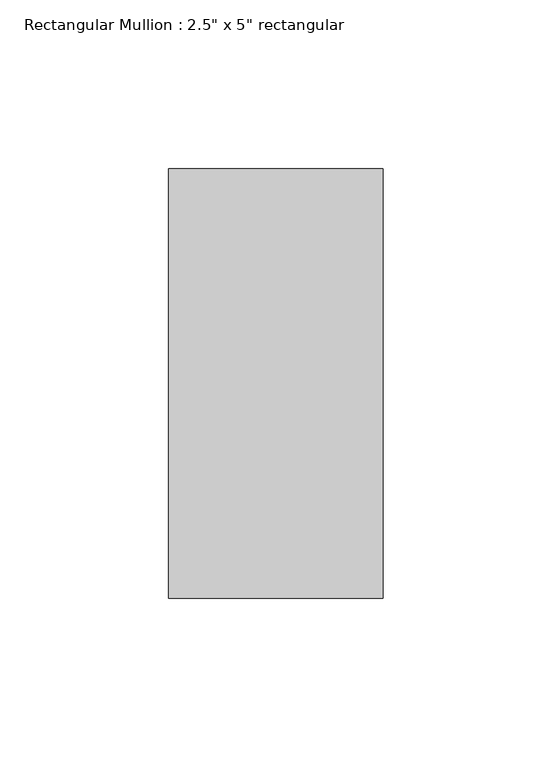
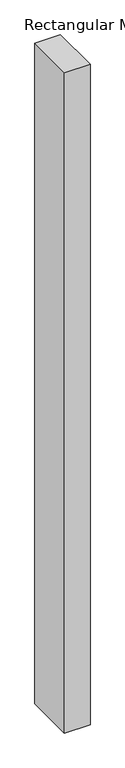
"""IFC4 building model written with IfcOpenShell, lengths in millimetres: member geometry."""

from ifc_helpers import new_model, si_unit, frame, origin, place, context, project, spatial, polyline, outline, extrude, source, transform, mapped, element, save


def member_8f1d4e4f(model_context):
    return source(origin(), model_context, "Body", "SweptSolid", [
        extrude(outline(polyline([(31.75, 63.5), (31.75, -63.5), (-31.75, -63.5), (-31.75, 63.5), (31.75, 63.5)])), frame((0.0, 0.0, -1732.6965064), z_axis=(0.0, 0.0, 1.0), x_axis=(1.0, 0.0, 0.0)), (0.0, 0.0, 1.0), 1732.6965064),
    ])


if __name__ == "__main__":
    model = new_model("IFC4")
    model_context = context("Model", 3, world=origin())
    ifc_project = project(units=[si_unit("LENGTHUNIT", "METRE", prefix="MILLI")], contexts=[model_context])
    site = spatial("IfcSite", under=ifc_project)
    building = spatial("IfcBuilding", under=site)
    placement = place(None, origin())
    member_shape = member_8f1d4e4f(model_context)
    element("IfcMember", 1, ObjectType="Rectangular Mullion : 2.5\" x 5\" rectangular", at=placement, inside=building, context=model_context, shape_type="MappedRepresentation", body=[
        mapped(member_shape, transform((0.0, 0.0, 0.0), x_axis=(1.0, 0.0, 0.0), y_axis=(0.0, 1.0, 0.0), z_axis=(0.0, 0.0, 1.0))),
    ])
    save(model, "model.ifc")

# Revit data of these elements
# Type "Rectangular Mullion : 2.5\" x 5\" rectangular"
#   built-in parameter 1007304 = 0.416667 (stored number, unit not read)
#   built-in parameter 1007301 = 0.104167 (stored number, unit not read)
#   built-in parameter 1007300 = 0.104167 (stored number, unit not read)
# Element 1 (IfcMember, "Rectangular Mullion : 2.5\" x 5\" rectangular")
#   Materials on its faces: "Aluminum"
# Materials
#   "Aluminum": class "Metal", colour RGB 247 247 247, transparency 0, Description = "Aluminum 6061", Cost = 0
